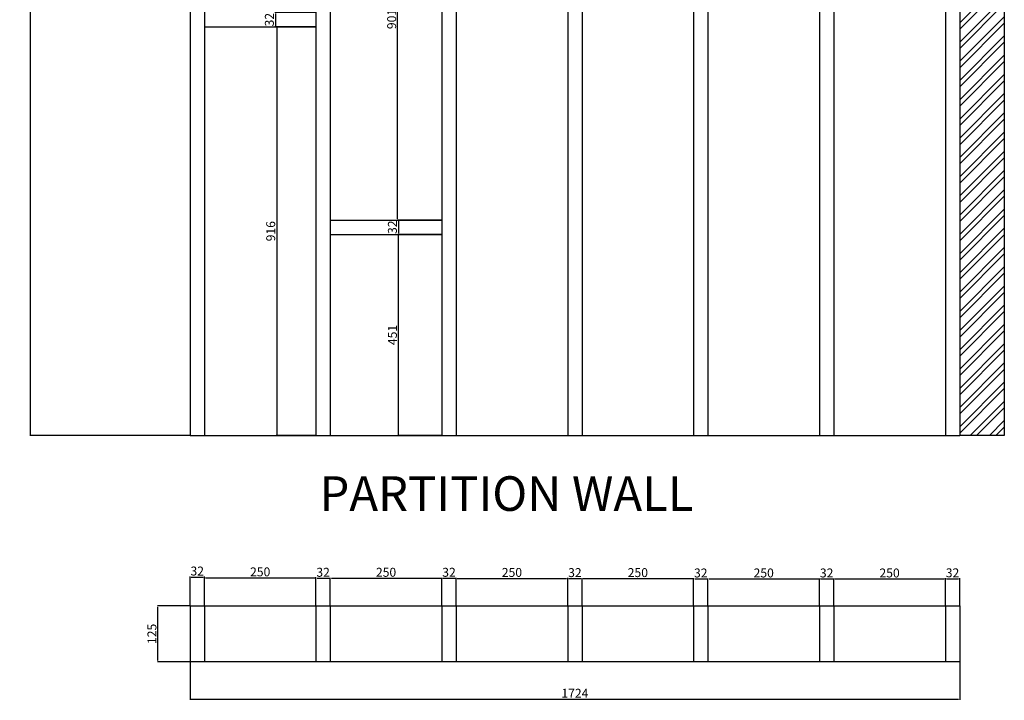
# Model space of a CAD drawing. Units: millimetres. Extents: x 1898 to 8115, y 727 to 4291.
# Tile 1 of 7: x 1898 to 4104, y 727 to 2252. Entities that reach past the tile are written whole.
import ezdxf

# ---------------------------------------------------------------- set-up
doc = ezdxf.new("R2010")
doc.units = ezdxf.units.MM
for name, color, linetype, lineweight in [('A-ANNO-DIMS', 2, 'Continuous', 18), ('A-ANNO-TEXT', 7, 'Continuous', 25), ('A-DETL', 7, 'Continuous', 25), ('A-DETL-PATT', 8, 'Continuous', 13)]:
    doc.layers.add(name, color=color, linetype=linetype, lineweight=lineweight)
doc.styles.get("Standard").update_dxf_attribs({"font": 'arial.ttf'})
doc.dimstyles.new('ISO-25', dxfattribs={"dimtxt": 20, "dimasz": 2.5, "dimexe": 1.25, "dimexo": 0.625, "dimtad": 1, "dimtxsty": 'Standard', "dimcen": 2.5, "dimadec": 0, "dimazin": 0, "dimtfac": 1, "dimtmove": 0, "dimatfit": 3, "dimfxl": 1, "dimarcsym": 0})

# ---------------------------------------------------------------- blocks, each defined once
blk = doc.blocks.new('*D1')
at = {"layer": 'A-ANNO-DIMS', "color": 0, "lineweight": -2, "transparency": 16777216}
for p, q in [((2279.1, 938.8), (2206.4, 938.8)), ((2207.6, 816.3), (2207.6, 936.3)), ((2279.1, 813.8), (2206.4, 813.8))]:
    blk.add_line(p, q, dxfattribs=at)
at = {"layer": 'A-ANNO-DIMS', "color": 0, "transparency": 16777216}
for points in [[(2207.2, 936.3), (2208.1, 936.3), (2207.6, 938.8)], [(2207.2, 816.3), (2208.1, 816.3), (2207.6, 813.8)]]:
    blk.add_solid(points, dxfattribs=at)
at = {"layer": 'Defpoints', "color": 0, "transparency": 16777216}
for p in [(2207.6, 938.8), (2279.7, 938.8), (2279.7, 813.8)]:
    blk.add_point(p, dxfattribs=at)
at = {"layer": 'A-ANNO-DIMS', "color": 0, "transparency": 16777216, "insert": (2196.8, 876.3), "char_height": 20, "attachment_point": 5, "rotation": 90}
blk.add_mtext('125', dxfattribs=at)
blk = doc.blocks.new('*D2')
at = {"layer": 'A-ANNO-DIMS', "color": 0, "lineweight": -2, "transparency": 16777216}
for p, q in [((2279.7, 939.5), (2279.7, 1004.9)), ((2282.2, 1003.6), (2309.2, 1003.6)), ((2311.7, 939.5), (2311.7, 1004.9))]:
    blk.add_line(p, q, dxfattribs=at)
at = {"layer": 'A-ANNO-DIMS', "color": 0, "transparency": 16777216}
for points in [[(2282.2, 1004), (2282.2, 1003.2), (2279.7, 1003.6)], [(2309.2, 1004), (2309.2, 1003.2), (2311.7, 1003.6)]]:
    blk.add_solid(points, dxfattribs=at)
at = {"layer": 'Defpoints', "color": 0, "transparency": 16777216}
for p in [(2311.7, 1003.6), (2279.7, 938.8), (2311.7, 938.8)]:
    blk.add_point(p, dxfattribs=at)
at = {"layer": 'A-ANNO-DIMS', "color": 0, "transparency": 16777216, "insert": (2295.7, 1014.5), "char_height": 20, "attachment_point": 5}
blk.add_mtext('32', dxfattribs=at)
blk = doc.blocks.new('*D3')
at = {"layer": 'A-ANNO-DIMS', "color": 0, "lineweight": -2, "transparency": 16777216}
for p, q in [((2311.7, 939.5), (2311.7, 1003)), ((2314.2, 1001.8), (2559.2, 1001.8)), ((2561.7, 939.5), (2561.7, 1003))]:
    blk.add_line(p, q, dxfattribs=at)
at = {"layer": 'A-ANNO-DIMS', "color": 0, "transparency": 16777216}
for points in [[(2314.2, 1002.2), (2314.2, 1001.3), (2311.7, 1001.8)], [(2559.2, 1002.2), (2559.2, 1001.3), (2561.7, 1001.8)]]:
    blk.add_solid(points, dxfattribs=at)
at = {"layer": 'Defpoints', "color": 0, "transparency": 16777216}
for p in [(2561.7, 1001.8), (2311.7, 938.8), (2561.7, 938.8)]:
    blk.add_point(p, dxfattribs=at)
at = {"layer": 'A-ANNO-DIMS', "color": 0, "transparency": 16777216, "insert": (2436.7, 1012.6), "char_height": 20, "attachment_point": 5}
blk.add_mtext('250', dxfattribs=at)
blk = doc.blocks.new('*D4')
at = {"layer": 'A-ANNO-DIMS', "color": 0, "lineweight": -2, "transparency": 16777216}
for p, q in [((2561.7, 939.5), (2561.7, 1002.1)), ((2564.2, 1000.9), (2591.2, 1000.9)), ((2593.7, 939.5), (2593.7, 1002.1))]:
    blk.add_line(p, q, dxfattribs=at)
at = {"layer": 'A-ANNO-DIMS', "color": 0, "transparency": 16777216}
for points in [[(2564.2, 1001.3), (2564.2, 1000.5), (2561.7, 1000.9)], [(2591.2, 1001.3), (2591.2, 1000.5), (2593.7, 1000.9)]]:
    blk.add_solid(points, dxfattribs=at)
at = {"layer": 'Defpoints', "color": 0, "transparency": 16777216}
for p in [(2593.7, 1000.9), (2561.7, 938.8), (2593.7, 938.8)]:
    blk.add_point(p, dxfattribs=at)
at = {"layer": 'A-ANNO-DIMS', "color": 0, "transparency": 16777216, "insert": (2577.7, 1011.7), "char_height": 20, "attachment_point": 5}
blk.add_mtext('32', dxfattribs=at)
blk = doc.blocks.new('*D5')
at = {"layer": 'A-ANNO-DIMS', "color": 0, "lineweight": -2, "transparency": 16777216}
for p, q in [((2593.7, 939.5), (2593.7, 1002.1)), ((2596.2, 1000.9), (2841.2, 1000.9)), ((2843.7, 939.5), (2843.7, 1002.1))]:
    blk.add_line(p, q, dxfattribs=at)
at = {"layer": 'A-ANNO-DIMS', "color": 0, "transparency": 16777216}
for points in [[(2596.2, 1001.3), (2596.2, 1000.5), (2593.7, 1000.9)], [(2841.2, 1001.3), (2841.2, 1000.5), (2843.7, 1000.9)]]:
    blk.add_solid(points, dxfattribs=at)
at = {"layer": 'Defpoints', "color": 0, "transparency": 16777216}
for p in [(2843.7, 1000.9), (2593.7, 938.8), (2843.7, 938.8)]:
    blk.add_point(p, dxfattribs=at)
at = {"layer": 'A-ANNO-DIMS', "color": 0, "transparency": 16777216, "insert": (2718.7, 1011.7), "char_height": 20, "attachment_point": 5}
blk.add_mtext('250', dxfattribs=at)
blk = doc.blocks.new('*D6')
at = {"layer": 'A-ANNO-DIMS', "color": 0, "lineweight": -2, "transparency": 16777216}
for p, q in [((2843.7, 939.5), (2843.7, 1002.1)), ((2846.2, 1000.9), (2873.2, 1000.9)), ((2875.7, 939.5), (2875.7, 1002.1))]:
    blk.add_line(p, q, dxfattribs=at)
at = {"layer": 'A-ANNO-DIMS', "color": 0, "transparency": 16777216}
for points in [[(2846.2, 1001.3), (2846.2, 1000.5), (2843.7, 1000.9)], [(2873.2, 1001.3), (2873.2, 1000.5), (2875.7, 1000.9)]]:
    blk.add_solid(points, dxfattribs=at)
at = {"layer": 'Defpoints', "color": 0, "transparency": 16777216}
for p in [(2875.7, 1000.9), (2843.7, 938.8), (2875.7, 938.8)]:
    blk.add_point(p, dxfattribs=at)
at = {"layer": 'A-ANNO-DIMS', "color": 0, "transparency": 16777216, "insert": (2859.7, 1011.7), "char_height": 20, "attachment_point": 5}
blk.add_mtext('32', dxfattribs=at)
blk = doc.blocks.new('*D7')
at = {"layer": 'A-ANNO-DIMS', "color": 0, "lineweight": -2, "transparency": 16777216}
for p, q in [((2875.7, 939.5), (2875.7, 1001.8)), ((2878.2, 1000.6), (3123.2, 1000.6)), ((3125.7, 939.5), (3125.7, 1001.8))]:
    blk.add_line(p, q, dxfattribs=at)
at = {"layer": 'A-ANNO-DIMS', "color": 0, "transparency": 16777216}
for points in [[(2878.2, 1001), (2878.2, 1000.1), (2875.7, 1000.6)], [(3123.2, 1001), (3123.2, 1000.1), (3125.7, 1000.6)]]:
    blk.add_solid(points, dxfattribs=at)
at = {"layer": 'Defpoints', "color": 0, "transparency": 16777216}
for p in [(3125.7, 1000.6), (2875.7, 938.8), (3125.7, 938.8)]:
    blk.add_point(p, dxfattribs=at)
at = {"layer": 'A-ANNO-DIMS', "color": 0, "transparency": 16777216, "insert": (3000.7, 1011.4), "char_height": 20, "attachment_point": 5}
blk.add_mtext('250', dxfattribs=at)
blk = doc.blocks.new('*D8')
at = {"layer": 'A-ANNO-DIMS', "color": 0, "lineweight": -2, "transparency": 16777216}
for p, q in [((3125.7, 939.5), (3125.7, 1001.4)), ((3128.2, 1000.2), (3155.2, 1000.2)), ((3157.7, 939.5), (3157.7, 1001.4))]:
    blk.add_line(p, q, dxfattribs=at)
at = {"layer": 'A-ANNO-DIMS', "color": 0, "transparency": 16777216}
for points in [[(3128.2, 1000.6), (3128.2, 999.8), (3125.7, 1000.2)], [(3155.2, 1000.6), (3155.2, 999.8), (3157.7, 1000.2)]]:
    blk.add_solid(points, dxfattribs=at)
at = {"layer": 'Defpoints', "color": 0, "transparency": 16777216}
for p in [(3157.7, 1000.2), (3125.7, 938.8), (3157.7, 938.8)]:
    blk.add_point(p, dxfattribs=at)
at = {"layer": 'A-ANNO-DIMS', "color": 0, "transparency": 16777216, "insert": (3141.7, 1011), "char_height": 20, "attachment_point": 5}
blk.add_mtext('32', dxfattribs=at)
blk = doc.blocks.new('*D9')
at = {"layer": 'A-ANNO-DIMS', "color": 0, "lineweight": -2, "transparency": 16777216}
for p, q in [((3157.7, 939.5), (3157.7, 1001.4)), ((3160.2, 1000.2), (3405.2, 1000.2)), ((3407.7, 939.5), (3407.7, 1001.4))]:
    blk.add_line(p, q, dxfattribs=at)
at = {"layer": 'A-ANNO-DIMS', "color": 0, "transparency": 16777216}
for points in [[(3160.2, 1000.6), (3160.2, 999.8), (3157.7, 1000.2)], [(3405.2, 1000.6), (3405.2, 999.8), (3407.7, 1000.2)]]:
    blk.add_solid(points, dxfattribs=at)
at = {"layer": 'Defpoints', "color": 0, "transparency": 16777216}
for p in [(3407.7, 1000.2), (3157.7, 938.8), (3407.7, 938.8)]:
    blk.add_point(p, dxfattribs=at)
at = {"layer": 'A-ANNO-DIMS', "color": 0, "transparency": 16777216, "insert": (3282.7, 1011), "char_height": 20, "attachment_point": 5}
blk.add_mtext('250', dxfattribs=at)
blk = doc.blocks.new('*D10')
at = {"layer": 'A-ANNO-DIMS', "color": 0, "lineweight": -2, "transparency": 16777216}
for p, q in [((3407.7, 939.5), (3407.7, 1000.6)), ((3410.2, 999.4), (3437.2, 999.4)), ((3439.7, 939.5), (3439.7, 1000.6))]:
    blk.add_line(p, q, dxfattribs=at)
at = {"layer": 'A-ANNO-DIMS', "color": 0, "transparency": 16777216}
for points in [[(3410.2, 999.8), (3410.2, 999), (3407.7, 999.4)], [(3437.2, 999.8), (3437.2, 999), (3439.7, 999.4)]]:
    blk.add_solid(points, dxfattribs=at)
at = {"layer": 'Defpoints', "color": 0, "transparency": 16777216}
for p in [(3439.7, 999.4), (3407.7, 938.8), (3439.7, 938.8)]:
    blk.add_point(p, dxfattribs=at)
at = {"layer": 'A-ANNO-DIMS', "color": 0, "transparency": 16777216, "insert": (3423.7, 1010.2), "char_height": 20, "attachment_point": 5}
blk.add_mtext('32', dxfattribs=at)
blk = doc.blocks.new('*D11')
at = {"layer": 'A-ANNO-DIMS', "color": 0, "lineweight": -2, "transparency": 16777216}
for p, q in [((3439.7, 939.5), (3439.7, 1000.6)), ((3442.2, 999.4), (3687.2, 999.4)), ((3689.7, 939.5), (3689.7, 1000.6))]:
    blk.add_line(p, q, dxfattribs=at)
at = {"layer": 'A-ANNO-DIMS', "color": 0, "transparency": 16777216}
for points in [[(3442.2, 999.8), (3442.2, 999), (3439.7, 999.4)], [(3687.2, 999.8), (3687.2, 999), (3689.7, 999.4)]]:
    blk.add_solid(points, dxfattribs=at)
at = {"layer": 'Defpoints', "color": 0, "transparency": 16777216}
for p in [(3689.7, 999.4), (3439.7, 938.8), (3689.7, 938.8)]:
    blk.add_point(p, dxfattribs=at)
at = {"layer": 'A-ANNO-DIMS', "color": 0, "transparency": 16777216, "insert": (3564.7, 1010.2), "char_height": 20, "attachment_point": 5}
blk.add_mtext('250', dxfattribs=at)
blk = doc.blocks.new('*D12')
at = {"layer": 'A-ANNO-DIMS', "color": 0, "lineweight": -2, "transparency": 16777216}
for p, q in [((3689.7, 939.5), (3689.7, 1000.6)), ((3692.2, 999.4), (3719.2, 999.4)), ((3721.7, 939.5), (3721.7, 1000.6))]:
    blk.add_line(p, q, dxfattribs=at)
at = {"layer": 'A-ANNO-DIMS', "color": 0, "transparency": 16777216}
for points in [[(3692.2, 999.8), (3692.2, 999), (3689.7, 999.4)], [(3719.2, 999.8), (3719.2, 999), (3721.7, 999.4)]]:
    blk.add_solid(points, dxfattribs=at)
at = {"layer": 'Defpoints', "color": 0, "transparency": 16777216}
for p in [(3721.7, 999.4), (3689.7, 938.8), (3721.7, 938.8)]:
    blk.add_point(p, dxfattribs=at)
at = {"layer": 'A-ANNO-DIMS', "color": 0, "transparency": 16777216, "insert": (3705.7, 1010.2), "char_height": 20, "attachment_point": 5}
blk.add_mtext('32', dxfattribs=at)
blk = doc.blocks.new('*D13')
at = {"layer": 'A-ANNO-DIMS', "color": 0, "lineweight": -2, "transparency": 16777216}
for p, q in [((3721.7, 939.5), (3721.7, 1000.6)), ((3724.2, 999.4), (3969.2, 999.4)), ((3971.7, 939.5), (3971.7, 1000.6))]:
    blk.add_line(p, q, dxfattribs=at)
at = {"layer": 'A-ANNO-DIMS', "color": 0, "transparency": 16777216}
for points in [[(3724.2, 999.8), (3724.2, 999), (3721.7, 999.4)], [(3969.2, 999.8), (3969.2, 999), (3971.7, 999.4)]]:
    blk.add_solid(points, dxfattribs=at)
at = {"layer": 'Defpoints', "color": 0, "transparency": 16777216}
for p in [(3971.7, 999.4), (3721.7, 938.8), (3971.7, 938.8)]:
    blk.add_point(p, dxfattribs=at)
at = {"layer": 'A-ANNO-DIMS', "color": 0, "transparency": 16777216, "insert": (3846.7, 1010.2), "char_height": 20, "attachment_point": 5}
blk.add_mtext('250', dxfattribs=at)
blk = doc.blocks.new('*D14')
at = {"layer": 'A-ANNO-DIMS', "color": 0, "lineweight": -2, "transparency": 16777216}
for p, q in [((3971.7, 939.5), (3971.7, 1000.9)), ((3974.2, 999.7), (4001.2, 999.7)), ((4003.7, 939.5), (4003.7, 1000.9))]:
    blk.add_line(p, q, dxfattribs=at)
at = {"layer": 'A-ANNO-DIMS', "color": 0, "transparency": 16777216}
for points in [[(3974.2, 1000.1), (3974.2, 999.3), (3971.7, 999.7)], [(4001.2, 1000.1), (4001.2, 999.3), (4003.7, 999.7)]]:
    blk.add_solid(points, dxfattribs=at)
at = {"layer": 'Defpoints', "color": 0, "transparency": 16777216}
for p in [(4003.7, 999.7), (3971.7, 938.8), (4003.7, 938.8)]:
    blk.add_point(p, dxfattribs=at)
at = {"layer": 'A-ANNO-DIMS', "color": 0, "transparency": 16777216, "insert": (3987.7, 1010.5), "char_height": 20, "attachment_point": 5}
blk.add_mtext('32', dxfattribs=at)
blk = doc.blocks.new('*D15')
at = {"layer": 'A-ANNO-DIMS', "color": 0, "lineweight": -2, "transparency": 16777216}
for p, q in [((2279.7, 813.2), (2279.7, 728.6)), ((4003.7, 813.2), (4003.7, 728.6)), ((2282.2, 729.9), (4001.2, 729.9))]:
    blk.add_line(p, q, dxfattribs=at)
at = {"layer": 'A-ANNO-DIMS', "color": 0, "transparency": 16777216}
for points in [[(2282.2, 730.3), (2282.2, 729.5), (2279.7, 729.9)], [(4001.2, 730.3), (4001.2, 729.5), (4003.7, 729.9)]]:
    blk.add_solid(points, dxfattribs=at)
at = {"layer": 'Defpoints', "color": 0, "transparency": 16777216}
for p in [(2279.7, 813.8), (4003.7, 813.8), (4003.7, 729.9)]:
    blk.add_point(p, dxfattribs=at)
at = {"layer": 'A-ANNO-DIMS', "color": 0, "transparency": 16777216, "insert": (3141.7, 740.6), "char_height": 20, "attachment_point": 5}
blk.add_mtext('1724', dxfattribs=at)
blk = doc.blocks.new('*D16')
at = {"layer": 'A-ANNO-DIMS', "color": 0, "lineweight": -2, "transparency": 16777216}
for p, q in [((2279.1, 4120.5), (1920.7, 4120.5)), ((1921.9, 1323), (1921.9, 4118)), ((2279.1, 1320.5), (1920.7, 1320.5))]:
    blk.add_line(p, q, dxfattribs=at)
at = {"layer": 'A-ANNO-DIMS', "color": 0, "transparency": 16777216}
for points in [[(1921.5, 4118), (1922.3, 4118), (1921.9, 4120.5)], [(1921.5, 1323), (1922.3, 1323), (1921.9, 1320.5)]]:
    blk.add_solid(points, dxfattribs=at)
at = {"layer": 'Defpoints', "color": 0, "transparency": 16777216}
for p in [(1921.9, 4120.5), (2279.7, 4120.5), (2279.7, 1320.5)]:
    blk.add_point(p, dxfattribs=at)
at = {"layer": 'A-ANNO-DIMS', "color": 0, "transparency": 16777216, "insert": (1911.1, 2720.5), "char_height": 20, "attachment_point": 5, "rotation": 90}
blk.add_mtext('2800', dxfattribs=at)
blk = doc.blocks.new('*D33')
at = {"layer": 'A-ANNO-DIMS', "color": 0, "lineweight": -2, "transparency": 16777216}
for p, q in [((2561.1, 2268.5), (2469.5, 2268.5)), ((2470.7, 2266), (2470.7, 2239)), ((2561.1, 2236.5), (2469.5, 2236.5))]:
    blk.add_line(p, q, dxfattribs=at)
at = {"layer": 'A-ANNO-DIMS', "color": 0, "transparency": 16777216}
for points in [[(2470.3, 2266), (2471.2, 2266), (2470.7, 2268.5)], [(2470.3, 2239), (2471.2, 2239), (2470.7, 2236.5)]]:
    blk.add_solid(points, dxfattribs=at)
at = {"layer": 'Defpoints', "color": 0, "transparency": 16777216}
for p in [(2561.7, 2268.5), (2470.7, 2236.5), (2561.7, 2236.5)]:
    blk.add_point(p, dxfattribs=at)
at = {"layer": 'A-ANNO-DIMS', "color": 0, "transparency": 16777216, "insert": (2459.9, 2252.5), "char_height": 20, "attachment_point": 5, "rotation": 90}
blk.add_mtext('32', dxfattribs=at)
blk = doc.blocks.new('*D34')
at = {"layer": 'A-ANNO-DIMS', "color": 0, "lineweight": -2, "transparency": 16777216}
for p, q in [((2561.1, 2236.5), (2472.5, 2236.5)), ((2473.7, 2234), (2473.7, 1323)), ((2561.1, 1320.5), (2472.5, 1320.5))]:
    blk.add_line(p, q, dxfattribs=at)
at = {"layer": 'A-ANNO-DIMS', "color": 0, "transparency": 16777216}
for points in [[(2473.3, 2234), (2474.1, 2234), (2473.7, 2236.5)], [(2473.3, 1323), (2474.1, 1323), (2473.7, 1320.5)]]:
    blk.add_solid(points, dxfattribs=at)
at = {"layer": 'Defpoints', "color": 0, "transparency": 16777216}
for p in [(2561.7, 2236.5), (2473.7, 1320.5), (2561.7, 1320.5)]:
    blk.add_point(p, dxfattribs=at)
at = {"layer": 'A-ANNO-DIMS', "color": 0, "transparency": 16777216, "insert": (2462.9, 1778.5), "char_height": 20, "attachment_point": 5, "rotation": 90}
blk.add_mtext('916', dxfattribs=at)
blk = doc.blocks.new('*D35')
at = {"layer": 'A-ANNO-DIMS', "color": 0, "lineweight": -2, "transparency": 16777216}
for p, q in [((2843.1, 1771.5), (2745.1, 1771.5)), ((2746.3, 1323), (2746.3, 1769)), ((2843.1, 1320.5), (2745.1, 1320.5))]:
    blk.add_line(p, q, dxfattribs=at)
at = {"layer": 'A-ANNO-DIMS', "color": 0, "transparency": 16777216}
for points in [[(2745.9, 1769), (2746.7, 1769), (2746.3, 1771.5)], [(2745.9, 1323), (2746.7, 1323), (2746.3, 1320.5)]]:
    blk.add_solid(points, dxfattribs=at)
at = {"layer": 'Defpoints', "color": 0, "transparency": 16777216}
for p in [(2746.3, 1771.5), (2843.7, 1771.5), (2843.7, 1320.5)]:
    blk.add_point(p, dxfattribs=at)
at = {"layer": 'A-ANNO-DIMS', "color": 0, "transparency": 16777216, "insert": (2735.5, 1546), "char_height": 20, "attachment_point": 5, "rotation": 90}
blk.add_mtext('451', dxfattribs=at)
blk = doc.blocks.new('*D36')
at = {"layer": 'A-ANNO-DIMS', "color": 0, "lineweight": -2, "transparency": 16777216}
for p, q in [((2843.1, 1803.5), (2745.1, 1803.5)), ((2746.3, 1801), (2746.3, 1774)), ((2843.1, 1771.5), (2745.1, 1771.5))]:
    blk.add_line(p, q, dxfattribs=at)
at = {"layer": 'A-ANNO-DIMS', "color": 0, "transparency": 16777216}
for points in [[(2745.9, 1801), (2746.7, 1801), (2746.3, 1803.5)], [(2745.9, 1774), (2746.7, 1774), (2746.3, 1771.5)]]:
    blk.add_solid(points, dxfattribs=at)
at = {"layer": 'Defpoints', "color": 0, "transparency": 16777216}
for p in [(2843.7, 1803.5), (2746.3, 1771.5), (2843.7, 1771.5)]:
    blk.add_point(p, dxfattribs=at)
at = {"layer": 'A-ANNO-DIMS', "color": 0, "transparency": 16777216, "insert": (2735.5, 1787.5), "char_height": 20, "attachment_point": 5, "rotation": 90}
blk.add_mtext('32', dxfattribs=at)
blk = doc.blocks.new('*D37')
at = {"layer": 'A-ANNO-DIMS', "color": 0, "lineweight": -2, "transparency": 16777216}
for p, q in [((2843.1, 2704.5), (2743.4, 2704.5)), ((2744.7, 1806), (2744.7, 2702)), ((2843.1, 1803.5), (2743.4, 1803.5))]:
    blk.add_line(p, q, dxfattribs=at)
at = {"layer": 'A-ANNO-DIMS', "color": 0, "transparency": 16777216}
for points in [[(2744.3, 2702), (2745.1, 2702), (2744.7, 2704.5)], [(2744.3, 1806), (2745.1, 1806), (2744.7, 1803.5)]]:
    blk.add_solid(points, dxfattribs=at)
at = {"layer": 'Defpoints', "color": 0, "transparency": 16777216}
for p in [(2744.7, 2704.5), (2843.7, 2704.5), (2843.7, 1803.5)]:
    blk.add_point(p, dxfattribs=at)
at = {"layer": 'A-ANNO-DIMS', "color": 0, "transparency": 16777216, "insert": (2733.8, 2254), "char_height": 20, "attachment_point": 5, "rotation": 90}
blk.add_mtext('901', dxfattribs=at)

msp = doc.modelspace()

# ---------------------------------------------------------------- hatches: boundary and pattern name
at = {"layer": 'A-DETL-PATT'}
h = msp.add_hatch(dxfattribs=at)
h.set_pattern_fill('ANSI32', color=256, scale=3.2)
h.set_pattern_definition([(45, (132, 2037.696), (-21.55261, 21.55261), []), (45, (146.368, 2037.696), (-21.55261, 21.55261), [])])
h.paths.add_polyline_path([(4003.701, 1320.491), (4103.701, 1320.491), (4103.701, 4120.491), (4003.701, 4120.491)])

# ---------------------------------------------------------------- linework, layer by layer
at = {"layer": 'A-DETL'}
for p, q in [((2279.701, 4120.491), (2279.701, 1320.491)), ((2843.701, 4120.491), (2843.701, 1320.491)), ((2875.701, 4120.491), (2875.701, 1320.491)), ((3407.701, 4106.462), (3407.701, 1320.491)), ((3971.701, 4120.491), (3971.701, 1320.491)), ((4003.701, 4120.491), (4003.701, 1320.491)), ((4103.701, 4120.491), (4103.701, 1320.491)), ((3125.701, 4087.257), (3125.701, 1320.491)), ((3439.701, 4083.546), (3439.701, 1320.491)), ((3689.701, 4096.592), (3689.701, 1320.491)), ((3721.701, 4089.634), (3721.701, 1320.491)), ((2311.701, 4071.26), (2311.701, 1320.491)), ((2561.701, 4071.663), (2561.701, 1320.491)), ((2593.701, 4077.96), (2593.701, 1320.491)), ((3157.701, 4070.861), (3157.701, 1320.491)), ((2311.701, 2236.491), (2561.701, 2236.491)), ((2593.701, 1803.491), (2843.701, 1803.491)), ((2593.701, 1771.491), (2843.701, 1771.491)), ((2279.701, 1320.491), (4003.701, 1320.491)), ((4103.701, 1320.491), (4003.701, 1320.491)), ((2279.701, 938.841), (2279.701, 813.841)), ((2279.701, 938.841), (4003.701, 938.841)), ((2311.701, 938.841), (2311.701, 813.841)), ((2561.701, 938.841), (2561.701, 813.841)), ((2593.701, 938.841), (2593.701, 813.841)), ((2843.701, 938.841), (2843.701, 813.841)), ((2875.701, 938.841), (2875.701, 813.841)), ((3125.701, 938.841), (3125.701, 813.841)), ((3157.701, 938.841), (3157.701, 813.841)), ((3407.701, 938.841), (3407.701, 813.841)), ((3439.701, 938.841), (3439.701, 813.841)), ((3689.701, 938.841), (3689.701, 813.841)), ((3721.701, 938.841), (3721.701, 813.841)), ((3971.701, 938.841), (3971.701, 813.841)), ((4003.701, 938.841), (4003.701, 813.841)), ((4003.701, 938.841), (4003.701, 813.841)), ((4003.701, 813.841), (2279.701, 813.841))]:
    msp.add_line(p, q, dxfattribs=at)

# ---------------------------------------------------------------- texts
at = {"layer": 'A-ANNO-TEXT', "insert": (2569.548, 1229.443), "char_height": 77.51345, "attachment_point": 1}
msp.add_mtext_dynamic_manual_height_columns('PARTITION WALL', width=11536.24269, gutter_width=387.567, heights=[0], dxfattribs=at)

# ---------------------------------------------------------------- dimensions: what is measured, and where the dimension line sits
at = {"layer": 'A-ANNO-DIMS'}
for base, p1, p2, picture, middle in [((1921.926, 4120.491), (2279.701, 1320.491), (2279.701, 4120.491), '*D16', (1911.089, 2720.491)), ((2744.671, 2704.491), (2843.701, 1803.491), (2843.701, 2704.491), '*D37', (2733.834, 2253.991)), ((2470.75, 2236.491), (2561.701, 2268.491), (2561.701, 2236.491), '*D33', (2459.906, 2252.491)), ((2473.728, 1320.491), (2561.701, 2236.491), (2561.701, 1320.491), '*D34', (2462.892, 1778.491)), ((2746.317, 1771.491), (2843.701, 1803.491), (2843.701, 1771.491), '*D36', (2735.473, 1787.491)), ((2746.317, 1771.491), (2843.701, 1320.491), (2843.701, 1771.491), '*D35', (2735.48, 1545.991)), ((2207.636, 938.841), (2279.701, 813.841), (2279.701, 938.841), '*D1', (2196.8, 876.341))]:
    dim = msp.add_linear_dim(base=base, p1=p1, p2=p2, angle=90, dimstyle='ISO-25', override={"dimclrd": 0, "dimclre": 0, "dimclrt": 0}, dxfattribs=at)
    dim.commit()
    dim.dimension.update_dxf_attribs({"geometry": picture, "text_midpoint": middle})
for base, p1, p2, picture, middle in [((2311.701, 1003.619), (2279.701, 938.841), (2311.701, 938.841), '*D2', (2295.701, 1014.462)), ((2561.701, 1001.752), (2311.701, 938.841), (2561.701, 938.841), '*D3', (2436.701, 1012.589)), ((2593.701, 1000.894), (2561.701, 938.841), (2593.701, 938.841), '*D4', (2577.701, 1011.738)), ((2843.701, 1000.894), (2593.701, 938.841), (2843.701, 938.841), '*D5', (2718.701, 1011.731)), ((2875.701, 1000.894), (2843.701, 938.841), (2875.701, 938.841), '*D6', (2859.701, 1011.738)), ((3125.701, 1000.563), (2875.701, 938.841), (3125.701, 938.841), '*D7', (3000.701, 1011.399)), ((3157.701, 1000.175), (3125.701, 938.841), (3157.701, 938.841), '*D8', (3141.701, 1011.019)), ((3407.701, 1000.175), (3157.701, 938.841), (3407.701, 938.841), '*D9', (3282.701, 1011.012)), ((3439.701, 999.399), (3407.701, 938.841), (3439.701, 938.841), '*D10', (3423.701, 1010.242)), ((3689.701, 999.399), (3439.701, 938.841), (3689.701, 938.841), '*D11', (3564.701, 1010.236)), ((3721.701, 999.399), (3689.701, 938.841), (3721.701, 938.841), '*D12', (3705.701, 1010.242)), ((3971.701, 999.399), (3721.701, 938.841), (3971.701, 938.841), '*D13', (3846.701, 1010.236)), ((4003.701, 999.678), (3971.701, 938.841), (4003.701, 938.841), '*D14', (3987.701, 1010.521)), ((4003.701, 729.897), (2279.701, 813.841), (4003.701, 813.841), '*D15', (3141.701, 740.563))]:
    dim = msp.add_linear_dim(base=base, p1=p1, p2=p2, dimstyle='ISO-25', override={"dimclrd": 0, "dimclre": 0, "dimclrt": 0}, dxfattribs=at)
    dim.commit()
    dim.dimension.update_dxf_attribs({"geometry": picture, "text_midpoint": middle})

doc.saveas('drawing.dxf')
